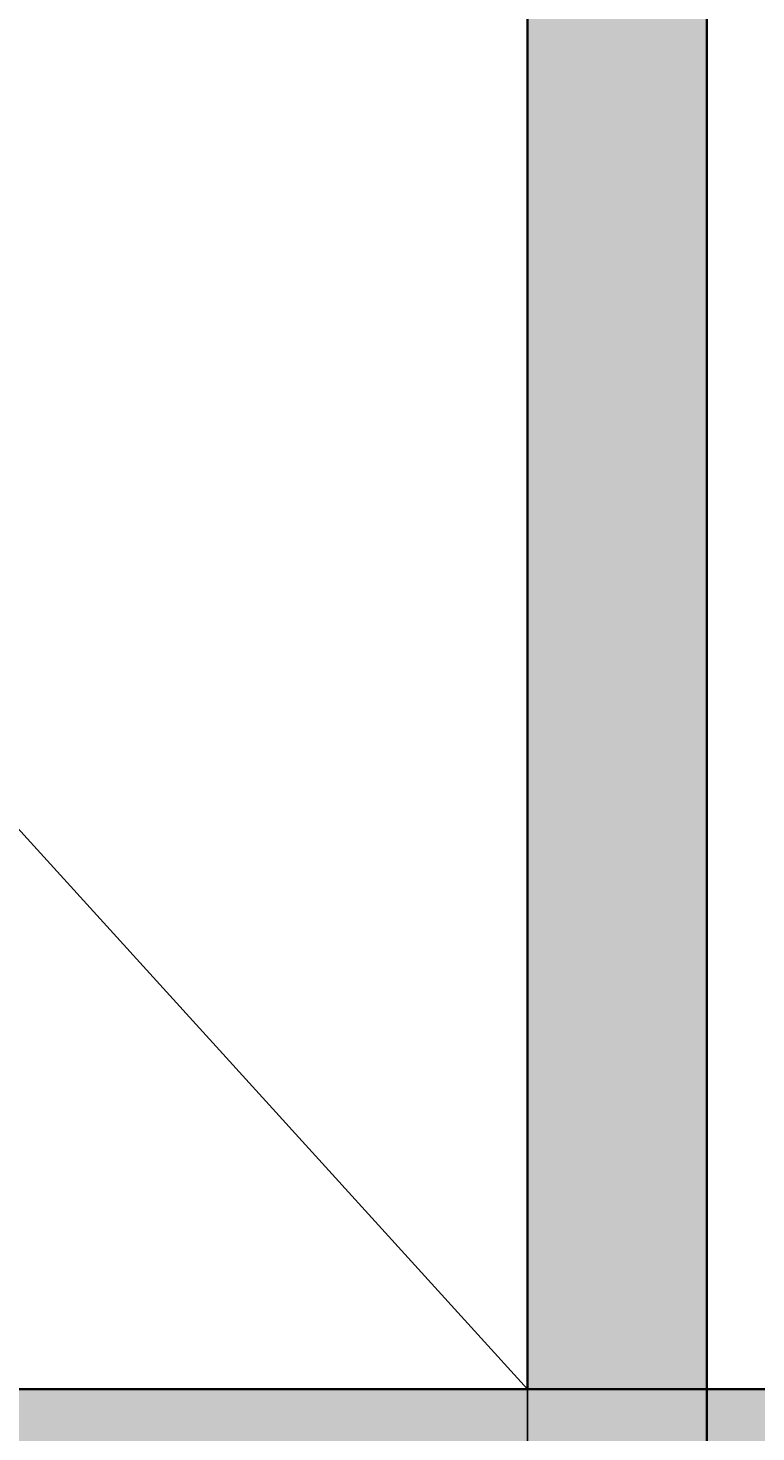
# Model space of a CAD drawing. Units: inches. Extents: x 1998 to 2588, y 1139 to 1977.
# Tile 36 of 134: x 2275 to 2293, y 1522 to 1557. Entities that reach past the tile are written whole.
import ezdxf

# ---------------------------------------------------------------- set-up
doc = ezdxf.new("R2010")
doc.units = ezdxf.units.IN
for name, color, linetype, lineweight in [('A-ANNO-DIMS', 2, 'Continuous', 18), ('A-FLOR-OPEN', 8, 'Continuous', 18), ('A-WALL-PATT', 252, 'Continuous', 13), ('WALL', 200, 'Continuous', 35)]:
    doc.layers.add(name, color=color, linetype=linetype, lineweight=lineweight)
doc.styles.get("Standard").update_dxf_attribs({"font": 'arial.ttf'})
doc.dimstyles.get("Standard").update_dxf_attribs({"dimtxt": 0.18, "dimasz": 0.18, "dimexe": 0.18, "dimexo": 0.0625, "dimgap": 0.09, "dimtad": 0, "dimtih": 1, "dimtoh": 1, "dimdec": 4, "dimzin": 0, "dimdsep": 46, "dimtxsty": 'Standard', "dimcen": 0.09, "dimadec": 0, "dimazin": 0, "dimtfac": 1, "dimtdec": 4, "dimtofl": 0, "dimtmove": 0, "dimatfit": 3, "dimfxl": 1, "dimtolj": 1, "dimtzin": 0, "dimarcsym": 0})

# ---------------------------------------------------------------- blocks, each defined once
blk = doc.blocks.new('*D34')
at = {"layer": 'A-ANNO-DIMS', "color": 0, "lineweight": -2, "transparency": 16777216}
for p, q in [((2407.91, 1594.732), (1997.843, 1594.732)), ((1998.023, 1594.552), (1998.023, 1558.913)), ((1998.023, 1522.912), (1998.023, 1558.552)), ((2407.91, 1522.732), (1997.843, 1522.732))]:
    blk.add_line(p, q, dxfattribs=at)
at = {"layer": 'A-ANNO-DIMS', "color": 0, "transparency": 16777216}
for points in [[(1997.993, 1594.552), (1998.053, 1594.552), (1998.023, 1594.732)], [(1997.993, 1522.912), (1998.053, 1522.912), (1998.023, 1522.732)]]:
    blk.add_solid(points, dxfattribs=at)
at = {"layer": 'Defpoints', "color": 0, "transparency": 16777216}
for p in [(1998.023, 1594.732), (2407.973, 1594.732), (2407.973, 1522.732)]:
    blk.add_point(p, dxfattribs=at)
at = {"layer": 'A-ANNO-DIMS', "color": 0, "transparency": 16777216, "insert": (1998.023, 1558.732), "char_height": 0.18, "attachment_point": 5}
blk.add_mtext('\\A1;72', dxfattribs=at)
blk = doc.blocks.new('*D41')
at = {"layer": 'A-ANNO-DIMS', "color": 0, "lineweight": -2, "transparency": 16777216}
for p, q in [((2227.473, 1588.67), (2227.473, 1138.602)), ((2287.473, 1588.67), (2287.473, 1138.602)), ((2227.653, 1138.782), (2257.254, 1138.782)), ((2287.293, 1138.782), (2257.692, 1138.782))]:
    blk.add_line(p, q, dxfattribs=at)
at = {"layer": 'A-ANNO-DIMS', "color": 0, "transparency": 16777216}
for points in [[(2227.653, 1138.812), (2227.653, 1138.752), (2227.473, 1138.782)], [(2287.293, 1138.812), (2287.293, 1138.752), (2287.473, 1138.782)]]:
    blk.add_solid(points, dxfattribs=at)
at = {"layer": 'Defpoints', "color": 0, "transparency": 16777216}
for p in [(2227.473, 1588.732), (2287.473, 1588.732), (2287.473, 1138.782)]:
    blk.add_point(p, dxfattribs=at)
at = {"layer": 'A-ANNO-DIMS', "color": 0, "transparency": 16777216, "insert": (2257.473, 1138.782), "char_height": 0.18, "attachment_point": 5}
blk.add_mtext('\\A1;60', dxfattribs=at)
blk = doc.blocks.new('*D42')
at = {"layer": 'A-ANNO-DIMS', "color": 0, "lineweight": -2, "transparency": 16777216}
for p, q in [((2287.535, 1588.732), (2588.309, 1588.732)), ((2588.129, 1588.552), (2588.129, 1555.914)), ((2588.129, 1522.912), (2588.129, 1555.55)), ((2287.535, 1522.732), (2588.309, 1522.732))]:
    blk.add_line(p, q, dxfattribs=at)
at = {"layer": 'A-ANNO-DIMS', "color": 0, "transparency": 16777216}
for points in [[(2588.099, 1588.552), (2588.159, 1588.552), (2588.129, 1588.732)], [(2588.099, 1522.912), (2588.159, 1522.912), (2588.129, 1522.732)]]:
    blk.add_solid(points, dxfattribs=at)
at = {"layer": 'Defpoints', "color": 0, "transparency": 16777216}
for p in [(2287.473, 1588.732), (2588.129, 1588.732), (2287.473, 1522.732)]:
    blk.add_point(p, dxfattribs=at)
at = {"layer": 'A-ANNO-DIMS', "color": 0, "transparency": 16777216, "insert": (2588.129, 1555.732), "char_height": 0.18, "attachment_point": 5}
blk.add_mtext('\\A1;66', dxfattribs=at)

msp = doc.modelspace()

# ---------------------------------------------------------------- hatches: boundary and pattern name
at = {"layer": 'A-WALL-PATT'}
h = msp.add_hatch(color=256, dxfattribs=at)
h.dxf.hatch_style = 1
h.paths.add_polyline_path([(2222.9729, 1888.7324), (2099.4125, 1888.7324), (2099.4125, 1879.7324), (2222.9729, 1879.7324)])
h.paths.add_polyline_path([(2096.9729, 1868.3278), (2087.9729, 1868.3278), (2087.9729, 1775.637), (2096.9729, 1775.637)])
h.paths.add_polyline_path([(2227.4729, 1868.3278), (2222.9729, 1868.3278), (2222.9729, 1774.3318), (2227.4729, 1774.3318)])
h.paths.add_polyline_path([(2188.3019, 1759.7324), (2138.6074, 1759.7324), (2099.4125, 1759.7324), (2099.4125, 1755.2324), (2176.9729, 1755.2324), (2188.3019, 1755.2324)])
h.paths.add_polyline_path([(2087.9729, 1759.7324), (2059.4729, 1759.7324), (2059.4729, 1702.7324), (2087.9729, 1702.7324), (2087.9729, 1707.2324), (2063.9729, 1707.2324), (2063.9729, 1755.2324), (2087.9729, 1755.2324)])
h.paths.add_polyline_path([(2096.9729, 1755.2324), (2087.9729, 1755.2324), (2087.9729, 1707.2324), (2096.9729, 1707.2324)])
h.paths.add_polyline_path([(2187.0461, 1707.2324), (2105.9729, 1707.2324), (2096.9729, 1707.2324), (2087.9729, 1707.2324), (2087.9729, 1702.7324), (2105.9729, 1702.7324), (2114.9729, 1702.7324), (2187.0461, 1702.7324)])
h.paths.add_polyline_path([(2181.4729, 1719.2028), (2176.9729, 1719.2028), (2176.9729, 1707.2324), (2181.4729, 1707.2324)])
h.paths.add_polyline_path([(2216.0332, 1588.7324), (2114.9729, 1588.7324), (2105.9729, 1588.7324), (2105.9729, 1584.2324), (2216.0332, 1584.2324)])
h.paths.add_polyline_path([(2077.691, 1588.7324), (2061.4729, 1588.7324), (2061.4729, 1584.2324), (2077.691, 1584.2324)])
h.paths.add_polyline_path([(2105.9729, 1588.7324), (2098.0956, 1588.7324), (2098.0956, 1584.2324), (2105.9729, 1584.2324)])
h.paths.add_polyline_path([(2114.9729, 1596.2642), (2110.1012, 1596.2642), (2105.9729, 1596.2642), (2105.9729, 1588.7324), (2114.9729, 1588.7324)])
h.paths.add_polyline_path([(2114.9729, 1584.2324), (2105.9729, 1584.2324), (2105.9729, 1580.249), (2110.1012, 1580.249), (2114.9729, 1580.249)])
h.paths.add_polyline_path([(2114.9729, 1547.7716), (2110.1012, 1547.7716, -0.0318759), (2105.9729, 1548.035), (2105.9729, 1470.2324), (2108.3775, 1470.2324), (2108.3775, 1465.7324), (2186.2943, 1465.7324), (2186.2943, 1470.2324), (2114.9729, 1470.2324)])
h.paths.add_polyline_path([(2227.4729, 1584.2324), (2222.9729, 1584.2324), (2222.9729, 1486.137), (2227.4729, 1486.137)])
h.paths.add_polyline_path([(2295.4138, 1593.2324), (2227.4729, 1593.2324), (2227.4729, 1588.7324), (2295.4138, 1588.7324), (2295.4138, 1591.8729)])
h.paths.add_polyline_path([(2345.9729, 1627.1165), (2341.4729, 1627.1165), (2341.4729, 1593.2324), (2337.2869, 1593.2324), (2337.2869, 1591.8729), (2337.2869, 1588.7324), (2345.9729, 1588.7324)])
h.paths.add_polyline_path([(2291.9729, 1588.7324), (2287.4729, 1588.7324), (2287.4729, 1522.7324), (2291.9729, 1522.7324)])
h.paths.add_polyline_path([(2291.9729, 1522.7324), (2287.4729, 1522.7324), (2227.4729, 1522.7324), (2227.4729, 1518.2324), (2291.9729, 1518.2324)])
h.paths.add_polyline_path([(2295.7347, 1519.5919), (2295.7347, 1522.7324), (2291.9729, 1522.7324), (2291.9729, 1518.2324), (2295.7347, 1518.2324)])
h.paths.add_polyline_path([(2345.9729, 1522.7324), (2337.6078, 1522.7324), (2337.6078, 1519.5919), (2337.6078, 1518.2324), (2341.4729, 1518.2324), (2341.4729, 1488.5616), (2345.9729, 1488.5616)])
h.paths.add_polyline_path([(2345.9729, 1468.1569), (2341.4729, 1468.1569), (2341.4729, 1374.2324), (2227.4729, 1374.2324), (2227.4729, 1369.7324), (2345.9729, 1369.7324)])
h.paths.add_polyline_path([(2345.9729, 1369.7324), (2341.4729, 1369.7324), (2341.4729, 1362.2324), (2345.9729, 1362.2324)])
h.paths.add_polyline_path([(2345.9729, 1317.7324), (2345.9729, 1322.2324), (2341.4729, 1322.2324), (2341.4729, 1285.137), (2345.9729, 1285.137)], flags=17)
h.paths.add_polyline_path([(2356.2096, 1322.2324), (2345.9729, 1322.2324), (2345.9729, 1317.7324), (2356.2096, 1317.7324), (2356.2096, 1319.3088)], flags=17)
h.paths.add_polyline_path([(2393.9729, 1322.2324), (2375.6999, 1322.2324), (2375.6999, 1319.3088, -0.0202458), (2375.636, 1317.7324), (2393.9729, 1317.7324)], flags=17)
h.paths.add_polyline_path([(2398.4729, 1322.2324), (2393.9729, 1322.2324), (2393.9729, 1317.7324), (2393.9729, 1237.7324), (2345.9729, 1237.7324), (2345.9729, 1264.7324), (2341.4729, 1264.7324), (2341.4729, 1228.7324), (2393.9729, 1228.7324), (2482.7412, 1228.7324), (2482.7412, 1237.7324), (2398.4729, 1237.7324), (2398.4729, 1297.1029)])
h.paths.add_polyline_path([(2398.4729, 1362.2324), (2393.9729, 1362.2324), (2393.9729, 1357.7324), (2398.4729, 1357.7324)])
h.paths.add_polyline_path([(2345.9729, 1329.7549), (2341.4729, 1329.7549), (2341.4729, 1322.2324), (2345.9729, 1322.2324)])

# ---------------------------------------------------------------- linework, layer by layer
at = {"layer": 'A-FLOR-OPEN'}
msp.add_line((2227.4729, 1588.7324), (2287.4729, 1522.7324), dxfattribs=at)
at = {"layer": 'WALL'}
for p, q in [((2287.4729, 1522.7324), (2287.4729, 1588.7324)), ((2291.9729, 1518.2324), (2291.9729, 1588.7324)), ((2227.4729, 1522.7324), (2287.4729, 1522.7324)), ((2227.4729, 1522.7324), (2295.7347, 1522.7324))]:
    msp.add_line(p, q, dxfattribs=at)

# ---------------------------------------------------------------- dimensions: what is measured, and where the dimension line sits
at = {"layer": 'A-ANNO-DIMS'}
for base, p1, p2, picture, middle in [((1998.0229, 1594.7324), (2407.9729, 1522.7324), (2407.9729, 1594.7324), '*D34', (1998.0229, 1558.7324)), ((2588.1286, 1588.7324), (2287.4729, 1522.7324), (2287.4729, 1588.7324), '*D42', (2588.1286, 1555.7324))]:
    dim = msp.add_linear_dim(base=base, p1=p1, p2=p2, angle=90, dimstyle='Standard', override={"dimdec": 0, "dimlfac": 1, "dimrnd": 0, "dimzin": 0, "dimdsep": 46, "dimlunit": 2}, dxfattribs=at)
    dim.commit()
    dim.dimension.update_dxf_attribs({"geometry": picture, "text_midpoint": middle})
dim = msp.add_linear_dim(base=(2287.4729, 1138.7824), p1=(2227.4729, 1588.7324), p2=(2287.4729, 1588.7324), dimstyle='Standard', override={"dimdec": 0, "dimlfac": 1, "dimrnd": 0, "dimzin": 0, "dimdsep": 46, "dimlunit": 2}, dxfattribs=at)
dim.commit()
dim.dimension.update_dxf_attribs({"geometry": '*D41', "text_midpoint": (2257.4729, 1138.7824)})

doc.saveas('drawing.dxf')
